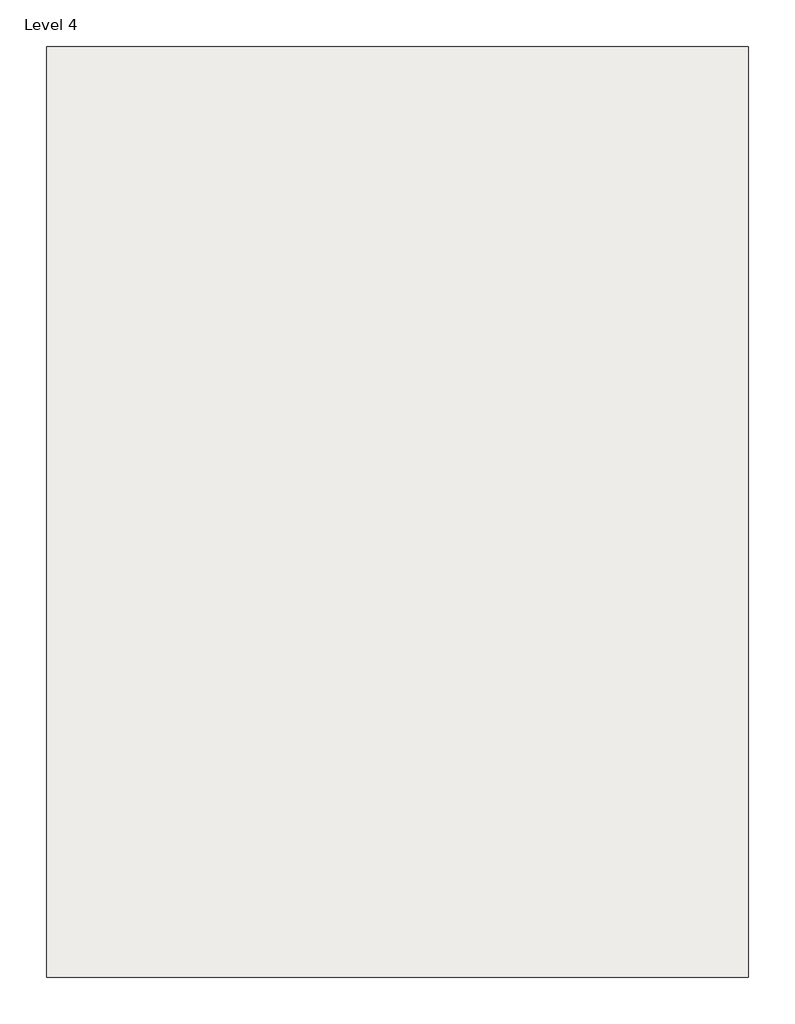
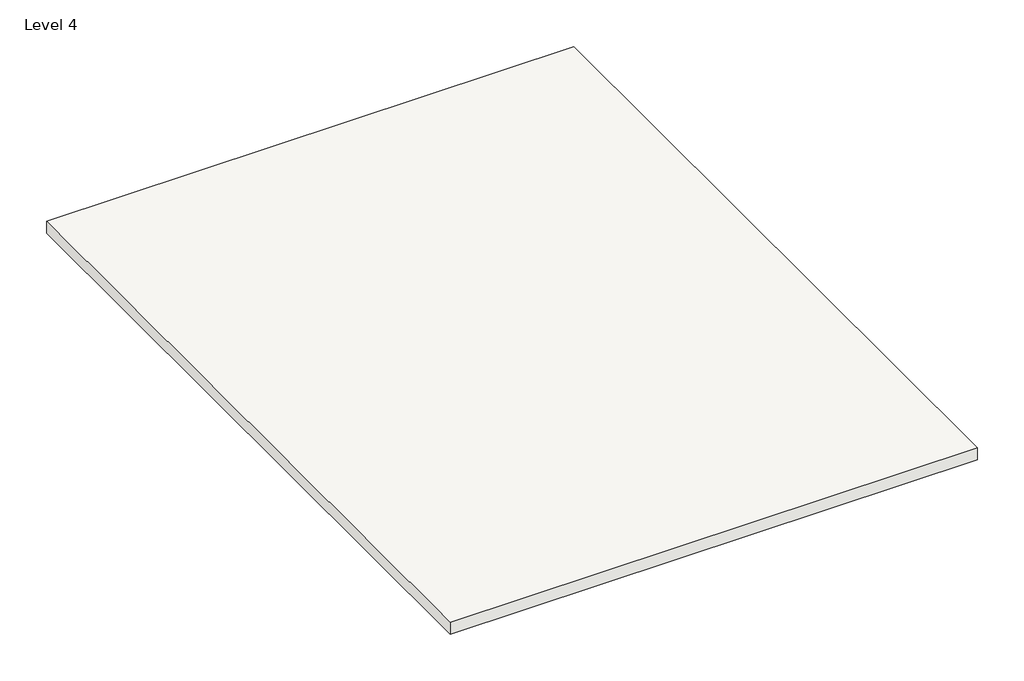
# One storey: 1 roof.
"""IFC4 building model written with IfcOpenShell, lengths in millimetres."""

from ifc_helpers import new_model, si_unit, frame, origin, place, context, project, spatial, polyline, outline, extrude, element, save

model = new_model("IFC4")

# Units and contexts
model_context = context("Model", 3, world=origin())
ifc_project = project(units=[si_unit("LENGTHUNIT", "METRE", prefix="MILLI")], contexts=[model_context])

# Site, building, storey
site = spatial("IfcSite", under=ifc_project)
building = spatial("IfcBuilding", under=site)
storey = spatial("IfcBuildingStorey", under=building, Name="Level 4", Elevation=6324.6)

# Roof
placement = place(None, origin())
element("IfcRoof", 1, ObjectType="Generic - 9\"", at=placement, inside=storey, context=model_context, shape_type="SweptSolid", body=[
    extrude(outline(polyline([(-10506.8128458, 14246.819734), (-1159.6128458, 14246.819734), (-1159.6128458, 1851.619734), (-10506.8128458, 1851.619734), (-10506.8128458, 14246.819734)])), frame((0.0, 0.0, 6324.6), z_axis=(0.0, 0.0, 1.0), x_axis=(1.0, 0.0, 0.0)), (0.0, 0.0, 1.0), 228.6),
])

save(model, "model.ifc")

# Revit data of these elements
# Type "Generic - 9\""
#   Assembly Code = "B1020"
#   Layers, outside or top first: 0' - 9" no material (function 1)
# Element 1 (IfcRoof, "Generic - 9\"")
#   built-in parameter 1001705 = 21.5 (stored number, unit not read)
#   built-in parameter 1001710 = 33615
#   Phase Created = New Construction
#   Materials on its faces: "Default Roof"
# Materials
#   "Default Roof": colour RGB 88 101 114, transparency 0
